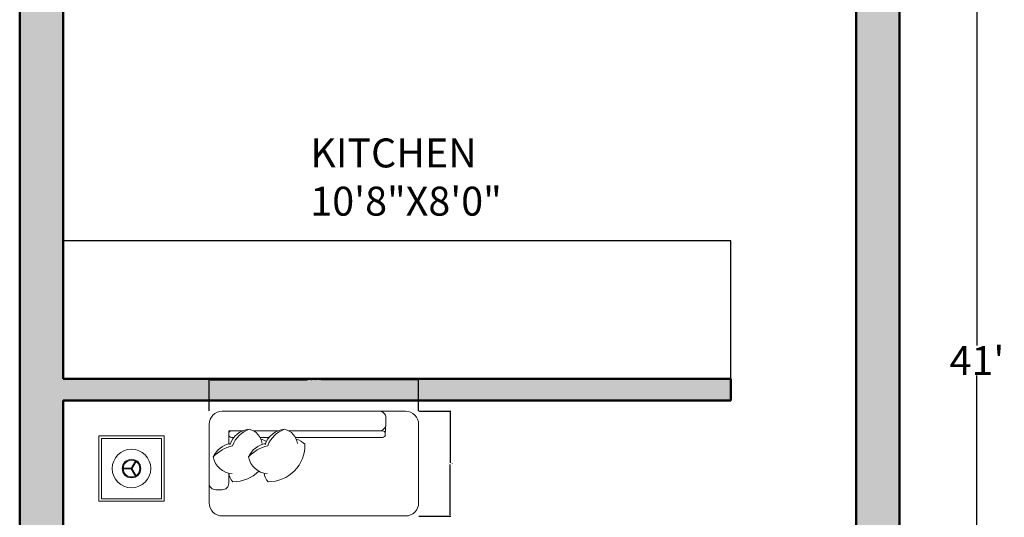
# Model space of a CAD drawing. Units: inches. Extents: x 3 to 485, y -522 to 42.
# Tile 2 of 6: x 30 to 235, y -264 to -161. Entities that reach past the tile are written whole.
import ezdxf

# ---------------------------------------------------------------- set-up
doc = ezdxf.new("R2010")
doc.units = ezdxf.units.IN
doc.header["$MEASUREMENT"] = 0
for name, color, linetype, lineweight in [('A-ANNO-DIMS', 2, 'Continuous', 18), ('A-AREA-IDEN', 7, 'Continuous', 18), ('A-FLOR-CASE', 8, 'Continuous', 25), ('A-FURN', 8, 'Continuous', 18), ('A-WALL', 7, 'Continuous', 50)]:
    doc.layers.add(name, color=color, linetype=linetype, lineweight=lineweight)
doc.layers.add('A-WALL-PATT', color=18, linetype='Continuous', lineweight=13, true_color=0x000000)
doc.styles.get("Standard").update_dxf_attribs({"font": 'arial.ttf'})
doc.dimstyles.get("Standard").update_dxf_attribs({"dimtxt": 0.18, "dimasz": 0.18, "dimexe": 0.18, "dimexo": 0.0625, "dimgap": 0.09, "dimtad": 0, "dimtih": 1, "dimtoh": 1, "dimdec": 0, "dimzin": 0, "dimdsep": 46, "dimlunit": 3, "dimtxsty": 'Standard', "dimcen": 0.09, "dimadec": 0, "dimazin": 0, "dimtfac": 1, "dimtdec": 0, "dimtofl": 0, "dimtmove": 0, "dimatfit": 3, "dimfxl": 1, "dimtolj": 1, "dimtzin": 0, "dimarcsym": 0})

# ---------------------------------------------------------------- blocks, each defined once
blk = doc.blocks.new('DAY BED1')
at = {"color": 0}
blk.add_line((0.3, 0.25), (0.225, 0.2549), dxfattribs=at)
blk.add_lwpolyline([(-0.3, 0, -0.414214), (-0.4, 0.1), (-0.4, 0.1, 0.317837), (-0.4, 0.1, -0.414214), (-0.4, 0.1), (-0.4, 0.1, 1.186185), (-0.4, 0.1, -0.414214), (-0.4, 0.1), (-0.4, 1.5, -0.414214), (-0.3, 1.6), (0.3, 1.6, -0.414214), (0.4, 1.5), (0.4, 0.1, -0.414214), (0.3, 0)], format="xyb", close=True, dxfattribs=at)
for points in [[(-0.0725, 1.45), (-0.15, 1.45, -0.414214), (-0.2, 1.5), (-0.2, 1.55, -0.414214), (-0.15, 1.6)], [(-0.0756, 1.4249, -0.356772), (0.0505, 1.5682, -0.249542), (0.1543, 1.4384, 9.61688)], [(0.0505, 1.5682, -0.14773), (0.1364, 1.422, -0.213343), (0.2624, 1.2931, -0.178662)], [(-0.0725, 1.4501, 0.165541), (-0.1386, 1.4192, 0.200231), (-0.0581, 1.2207, 0.121523)], [(0.1433, 1.4422, -0.306663), (0.2624, 1.2931, -0.30633), (0.1536, 1.1957, 0.872847)], [(0.25, 1.3448), (0.25, 1.45), (0.1517, 1.45, -0.414214)], [(0.2, 1.4118), (0.2, 1.43, -0.414214), (0.22, 1.45), (0.23, 1.45, -0.414214), (0.25, 1.43)], [(0.25, 1.43), (0.25, 1.3448, -0.414214)], [(-0.0756, 1.1556, -0.356772), (0.0505, 1.2988, -0.249542), (0.1543, 1.169, 9.61688)], [(0.0505, 1.2988, -0.14773), (0.1364, 1.1527, -0.213343), (0.2624, 1.0238, -0.178662)], [(0.1678, 1.1631, 0.071865), (0.1873, 1.205, -7.115464)], [(0.2, 1.1425), (0.2, 1.2113, -0.414214)], [(0.25, 1.2616), (0.25, 1.0755, -0.414214)], [(-0.0725, 1.1808, 0.165541), (-0.1386, 1.1498, 0.425989), (0.1479, 0.869, 0.121523), (0.1873, 0.9357, -7.115464)], [(0.1433, 1.1729, -0.306663), (0.2624, 1.0238, -0.30633), (0.1536, 0.9263, 0.872847)], [(0.25, 0.9923), (0.25, 0.2749, -0.414214), (0.23, 0.2549), (0.22, 0.2549, -0.414214), (0.2, 0.2749), (0.2, 0.9419, -0.414214)], [(0.25, 0.3775), (0.25, 0.3, 0.414214), (0.3, 0.25), (0.35, 0.25, 0.414214), (0.4, 0.3)]]:
    blk.add_lwpolyline(points, format="xyb", dxfattribs=at)
for points in [[(0.25, 1.0755), (0.25, 1.2616)], [(0.25, 0.3775), (0.25, 0.9923)]]:
    blk.add_lwpolyline(points, dxfattribs=at)
blk = doc.blocks.new('*D5')
at = {"layer": 'A-ANNO-DIMS', "color": 0, "lineweight": -2, "transparency": 16777216}
for p, q in [((212.85, 14), (229.02, 14)), ((228.84, 13.82), (228.84, -228.64)), ((228.84, -477.32), (228.84, -234.85)), ((212.85, -477.5), (229.02, -477.5))]:
    blk.add_line(p, q, dxfattribs=at)
at = {"layer": 'A-ANNO-DIMS', "color": 0, "transparency": 16777216}
for points in [[(228.81, 13.82), (228.87, 13.82), (228.84, 14)], [(228.81, -477.32), (228.87, -477.32), (228.84, -477.5)]]:
    blk.add_solid(points, dxfattribs=at)
at = {"layer": 'Defpoints', "color": 0, "transparency": 16777216}
for p in [(212.79, 14), (212.79, -477.5), (228.84, -477.5)]:
    blk.add_point(p, dxfattribs=at)
at = {"layer": 'A-ANNO-DIMS', "color": 0, "transparency": 16777216, "insert": (228.84, -231.75), "char_height": 6, "attachment_point": 5}
blk.add_mtext("\\A1;41'", dxfattribs=at)
blk = doc.blocks.new('LIVING-SIDE-TABLE')
for p, q in [((6.72, 6.83), (7.67, 8.49)), ((6.86, 6.75), (7.82, 8.41)), ((6.79, 6.87), (4.87, 6.87)), ((6.79, 6.7), (4.87, 6.7)), ((6.72, 6.75), (7.67, 5.09)), ((6.86, 6.83), (7.82, 5.17))]:
    blk.add_line(p, q)
at = {"ltscale": 0.03}
blk.add_lwpolyline([(13.58, 13.58), (13.58, 0), (0, 0), (0, 13.58)], close=True, dxfattribs=at)
blk.add_lwpolyline([(13.04, 0.54), (13.04, 13.04), (0.54, 13.04), (0.54, 0.54)], close=True)
for radius in [4, 1.92, 1.72]:
    blk.add_circle((6.79, 6.79), radius)
blk = doc.blocks.new('*D18')
at = {"layer": 'A-ANNO-DIMS', "color": 0, "lineweight": -2, "transparency": 16777216}
for p, q in [((69.59, -242.18), (69.59, -235.54)), ((69.77, -235.72), (89.89, -235.72)), ((112.86, -235.72), (92.75, -235.72)), ((113.04, -242.18), (113.04, -235.54))]:
    blk.add_line(p, q, dxfattribs=at)
at = {"layer": 'A-ANNO-DIMS', "color": 0, "transparency": 16777216}
for points in [[(69.77, -235.69), (69.77, -235.75), (69.59, -235.72)], [(112.86, -235.69), (112.86, -235.75), (113.04, -235.72)]]:
    blk.add_solid(points, dxfattribs=at)
at = {"layer": 'Defpoints', "color": 0, "transparency": 16777216}
for p in [(69.59, -235.72), (69.59, -242.24), (113.04, -242.24)]:
    blk.add_point(p, dxfattribs=at)
at = {"layer": 'A-ANNO-DIMS', "color": 0, "transparency": 16777216, "insert": (91.32, -235.72), "char_height": 0.18, "attachment_point": 5}
blk.add_mtext('\\A1;DAY BED 3\'-7 1/2" TYP.', dxfattribs=at)
blk = doc.blocks.new('*D19')
at = {"layer": 'A-ANNO-DIMS', "color": 0, "lineweight": -2, "transparency": 16777216}
for p, q in [((113.11, -242.24), (119.74, -242.24)), ((119.56, -242.42), (119.56, -252.92)), ((119.56, -263.79), (119.56, -253.29)), ((113.11, -263.97), (119.74, -263.97))]:
    blk.add_line(p, q, dxfattribs=at)
at = {"layer": 'A-ANNO-DIMS', "color": 0, "transparency": 16777216}
for points in [[(119.53, -242.42), (119.59, -242.42), (119.56, -242.24)], [(119.53, -263.79), (119.59, -263.79), (119.56, -263.97)]]:
    blk.add_solid(points, dxfattribs=at)
at = {"layer": 'Defpoints', "color": 0, "transparency": 16777216}
for p in [(113.04, -242.24), (119.56, -242.24), (113.04, -263.97)]:
    blk.add_point(p, dxfattribs=at)
at = {"layer": 'A-ANNO-DIMS', "color": 0, "transparency": 16777216, "insert": (119.56, -253.1), "char_height": 0.18, "attachment_point": 5}
blk.add_mtext('\\A1;1\'-9 1/2" TYP.', dxfattribs=at)

msp = doc.modelspace()

# ---------------------------------------------------------------- hatches: boundary and pattern name
at = {"layer": 'A-WALL-PATT'}
h = msp.add_hatch(color=256, dxfattribs=at)
h.dxf.hatch_style = 1
h.paths.add_polyline_path([(177.79, -240), (177.79, -235.5), (39.29, -235.5), (39.29, 5), (87.29, 5), (87.29, -53), (91.79, -53), (91.79, 5), (203.79, 5), (203.79, -477.5), (212.79, -477.5), (212.79, 14), (30.29, 14), (30.29, -477.5), (39.29, -477.5), (39.29, -388.5), (94.55, -388.5), (94.55, -384), (39.29, -384), (39.29, -240)])
h.paths.add_polyline_path([(142.75, -477.5), (142.75, -468.5), (82.75, -468.5), (82.75, -477.5)], flags=17)
h.paths.add_polyline_path([(63.29, -79), (63.29, -83.5), (87.29, -83.5), (89.54, -83.5), (91.79, -83.5), (91.79, -77), (87.29, -77), (87.29, -79)], flags=17)
h.paths.add_polyline_path([(177.79, -139.5), (177.79, -135), (91.79, -135), (87.29, -135), (87.29, -139.5), (91.79, -139.5)], flags=17)

# ---------------------------------------------------------------- linework, layer by layer
at = {"layer": 'A-FLOR-CASE'}
for p, q in [((177.79, -206.9), (39.29, -206.9)), ((177.79, -235.5), (177.79, -206.9))]:
    msp.add_line(p, q, dxfattribs=at)
at = {"layer": 'A-WALL'}
for p, q in [((30.29, 14), (30.29, -477.5)), ((212.79, 14), (212.79, -477.5)), ((39.29, 5), (39.29, -235.5)), ((203.79, 5), (203.79, -477.5)), ((39.29, -235.5), (177.79, -235.5)), ((177.79, -235.5), (177.79, -240)), ((39.29, -240), (177.79, -240)), ((39.29, -240), (39.29, -384))]:
    msp.add_line(p, q, dxfattribs=at)

# ---------------------------------------------------------------- block references
at = {"layer": 'A-FURN', "ltscale": 0.03, "xscale": 27.15874568996764, "yscale": 27.15874568996764, "zscale": 27.15874568996764, "rotation": 90}
msp.add_blockref('DAY BED1', (113.04, -253.1), dxfattribs=at)
at = {"layer": 'A-FURN'}
msp.add_blockref('LIVING-SIDE-TABLE', (46.69, -260.92), dxfattribs=at)

# ---------------------------------------------------------------- texts
at = {"layer": 'A-AREA-IDEN', "insert": (90.58, -185.69), "char_height": 6, "attachment_point": 1}
msp.add_mtext('KITCHEN\\P10\'8"X8\'0"', dxfattribs=at)

# ---------------------------------------------------------------- dimensions: what is measured, and where the dimension line sits
at = {"layer": 'A-ANNO-DIMS'}
dim = msp.add_linear_dim(base=(228.83525514, -477.49647159), p1=(212.79082571, 14.00352841), p2=(212.79082571, -477.49647159), angle=90, dimstyle='Standard', override={"dimtxt": 6, "dimclrd": 0, "dimclre": 0, "dimclrt": 0}, dxfattribs=at)
dim.commit()
dim.dimension.update_dxf_attribs({"geometry": '*D5', "text_midpoint": (228.83525514, -231.74647159)})
for base, p1, p2, angle, text, picture, middle in [((69.5908, -235.7228), (113.0448, -242.2409), (69.5908, -242.2409), 180, 'DAY BED <> TYP.', '*D18', (91.3178, -235.7228)), ((119.56, -242.24), (113.04, -263.97), (113.04, -242.24), 90, '<> TYP.', '*D19', (119.56, -253.1))]:
    dim = msp.add_linear_dim(base=base, p1=p1, p2=p2, angle=angle, text=text, dimstyle='Standard', override={"dimdec": 1, "dimlfac": 1, "dimrnd": 0, "dimzin": 1, "dimdsep": 46, "dimlunit": 4, "dimfrac": 2}, dxfattribs=at)
    dim.commit()
    dim.dimension.update_dxf_attribs({"geometry": picture, "text_midpoint": middle})

doc.saveas('drawing.dxf')
